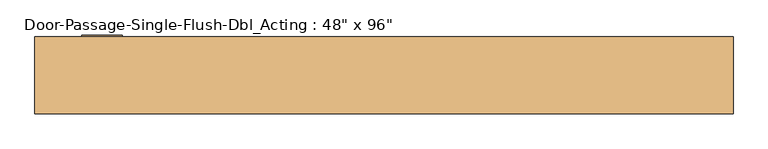
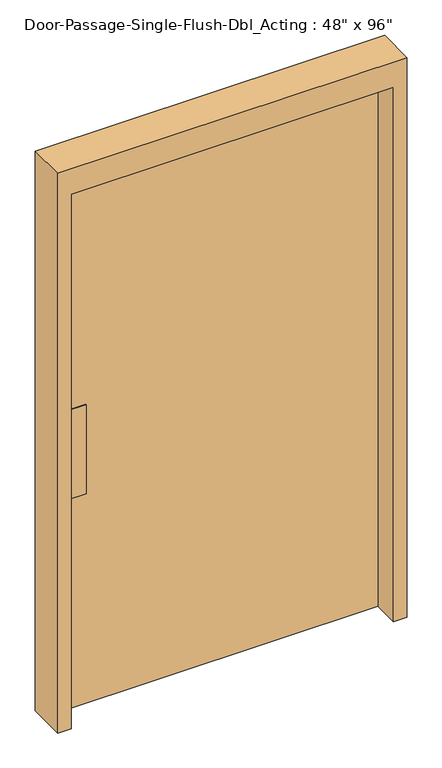
"""IFC4 building model written with IfcOpenShell, lengths in millimetres: door geometry."""

from ifc_helpers import new_model, si_unit, frame, origin, origin_with_axes, place, context, project, spatial, polyline, outline, extrude, source, transform, mapped, element, save


def door_15d3c954(model_context):
    return source(origin(), model_context, "Body", "SweptSolid", [
        extrude(outline(polyline([(-571.5, 34.925), (-571.5, 38.1), (-495.3, 38.1), (-495.3, 34.925), (-571.5, 34.925)])), frame((0.0, 0.0, 838.2), z_axis=(0.0, 0.0, 1.0), x_axis=(1.0, 0.0, 0.0)), (0.0, 0.0, 1.0), 355.6),
        extrude(outline(polyline([(-571.5, 85.725), (-495.3, 85.725), (-495.3, 82.55), (-571.5, 82.55), (-571.5, 85.725)])), frame((0.0, 0.0, 838.2), z_axis=(0.0, 0.0, 1.0), x_axis=(1.0, 0.0, 0.0)), (0.0, 0.0, 1.0), 355.6),
        extrude(outline(polyline([(0.0, 609.6), (0.0, 660.4), (2235.2, 660.4), (2235.2, -660.4), (0.0, -660.4), (0.0, -609.6), (2133.6, -609.6), (2133.6, 609.6), (0.0, 609.6)])), frame((0.0, -63.5, 0.0), z_axis=(0.0, 1.0, 0.0), x_axis=(0.0, 0.0, 1.0)), (0.0, 0.0, 1.0), 146.05),
        extrude(outline(polyline([(609.6, 38.1), (-609.6, 38.1), (-609.6, 82.55), (609.6, 82.55), (609.6, 38.1)])), origin_with_axes(), (0.0, 0.0, 1.0), 2133.6),
    ])


if __name__ == "__main__":
    model = new_model("IFC4")
    model_context = context("Model", 3, world=origin())
    ifc_project = project(units=[si_unit("LENGTHUNIT", "METRE", prefix="MILLI")], contexts=[model_context])
    site = spatial("IfcSite", under=ifc_project)
    building = spatial("IfcBuilding", under=site)
    placement = place(None, origin())
    door_shape = door_15d3c954(model_context)
    element("IfcDoor", 1, ObjectType="Door-Passage-Single-Flush-Dbl_Acting : 48\" x 96\"", at=placement, inside=building, context=model_context, shape_type="MappedRepresentation", body=[
        mapped(door_shape, transform((0.0, 0.0, 0.0), x_axis=(1.0, 0.0, 0.0), y_axis=(0.0, 1.0, 0.0), z_axis=(0.0, 0.0, 1.0))),
    ])
    save(model, "model.ifc")

# Revit data of these elements
# Type "Door-Passage-Single-Flush-Dbl_Acting : 48\" x 96\""
#   Type Mark = "12"
#   Assembly Code = "B2030200"
#   Analytic Construction = "Wooden"
#   Thickness = 0' - 1 3/4"
#   Thermal Resistance (R) = 2.5876 (h·ft²·°F)/BTU
#   Swing Angle [instance default] = 45.00°
#   Strike Height = 3' - 4"
#   Rough Width [instance default] = 4' - 4"
#   Rough Height [instance default] = 7' - 4"
#   MF Opening Height [instance default] = 0' - 4"
#   MF Opening Width [instance default] = 0' - 4"
#   Inset Calculate [instance default] = 0' - 4"
#   Masonry Inset [instance default] = 0' - 1"
#   Height = 7' - 0"
#   Width = 4' - 0"
#   Heat Transfer Coefficient (U) = 0.3865 BTU/(h·ft²·°F)
#   Masonry Frame Depth = 0' - 5 3/4"
#   Masonry Frame [instance default] = yes
#   Function = 1
#   Dry Wall Frame [instance default] = no
#   Panel Material = Wood - Birch
#   Frame Material = Metal - Paint Finish - Grey
#   Door Handle Material = Aluminum
#   Visual Light Transmittance = 0
#   Solar Heat Gain Coefficient = 0
#   Wall Closure = (empty or 0)
# Element 1 (IfcDoor, "Door-Passage-Single-Flush-Dbl_Acting : 48\" x 96\"")
#   Materials on its faces: "Aluminum", "Metal - Paint Finish - Grey", "Wood - Birch"
# Materials
#   "Wood - Birch": class "Wood", colour RGB 166 116 52, transparency 0, Cost = 0
#   "Metal - Paint Finish - Grey": class "Paint", colour RGB 104 104 104, transparency 0, Cost = 0
#   "Aluminum": class "Metal", colour RGB 247 247 247, transparency 0, Description = "Aluminum 6061", Cost = 0
